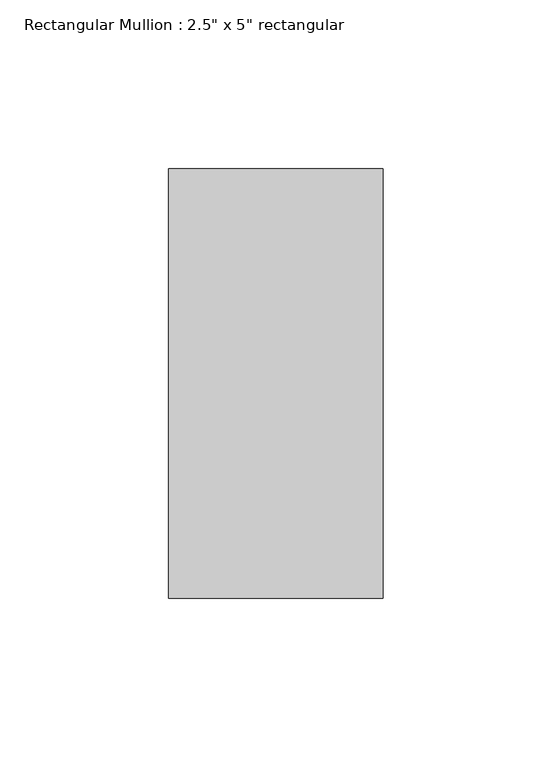
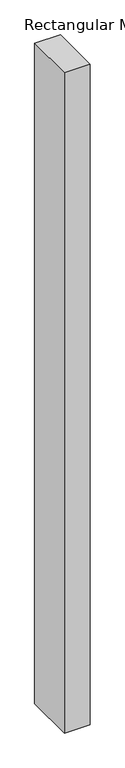
"""IFC4 building model written with IfcOpenShell, lengths in millimetres: member geometry."""

from ifc_helpers import new_model, si_unit, frame, origin, place, context, project, spatial, polyline, outline, extrude, source, transform, mapped, element, save


def member_106fc096(model_context):
    return source(origin(), model_context, "Body", "SweptSolid", [
        extrude(outline(polyline([(0.0, 63.5), (0.0, -63.5), (-63.5, -63.5), (-63.5, 63.5), (0.0, 63.5)])), frame((0.0, 0.0, -1719.9882445), z_axis=(0.0, 0.0, 1.0), x_axis=(1.0, 0.0, 0.0)), (0.0, 0.0, 1.0), 1719.9882445),
    ])


if __name__ == "__main__":
    model = new_model("IFC4")
    model_context = context("Model", 3, world=origin())
    ifc_project = project(units=[si_unit("LENGTHUNIT", "METRE", prefix="MILLI")], contexts=[model_context])
    site = spatial("IfcSite", under=ifc_project)
    building = spatial("IfcBuilding", under=site)
    placement = place(None, origin())
    member_shape = member_106fc096(model_context)
    element("IfcMember", 1, ObjectType="Rectangular Mullion : 2.5\" x 5\" rectangular", at=placement, inside=building, context=model_context, shape_type="MappedRepresentation", body=[
        mapped(member_shape, transform((0.0, 0.0, 0.0), x_axis=(1.0, 0.0, 0.0), y_axis=(0.0, 1.0, 0.0), z_axis=(0.0, 0.0, 1.0))),
    ])
    save(model, "model.ifc")

# Revit data of these elements
# Type "Rectangular Mullion : 2.5\" x 5\" rectangular"
#   built-in parameter 1007304 = 0.416667 (stored number, unit not read)
#   built-in parameter 1007301 = 0.104167 (stored number, unit not read)
#   built-in parameter 1007300 = 0.104167 (stored number, unit not read)
# Element 1 (IfcMember, "Rectangular Mullion : 2.5\" x 5\" rectangular")
#   Materials on its faces: "Aluminum"
# Materials
#   "Aluminum": class "Metal", colour RGB 247 247 247, transparency 0, Description = "Aluminum 6061", Cost = 0
